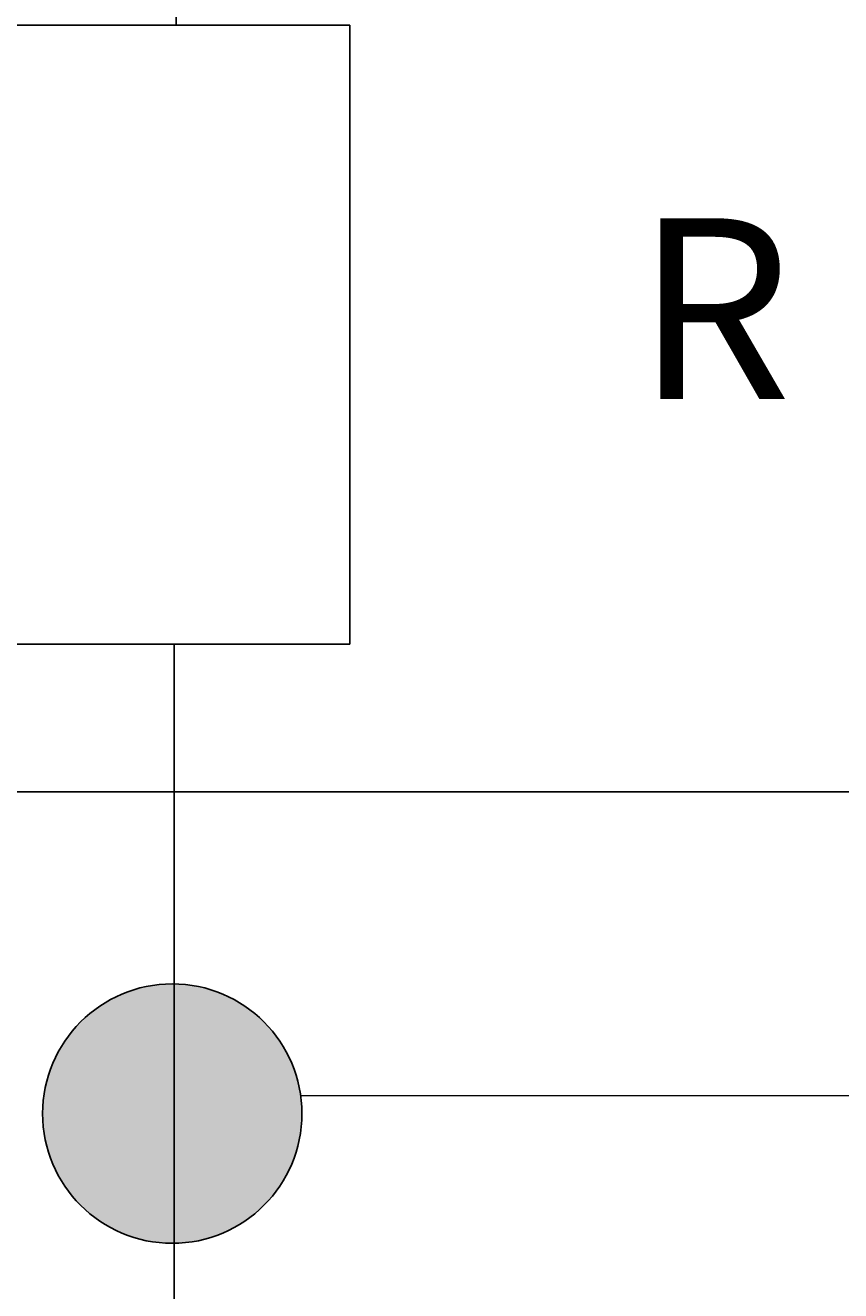
# Model space of a CAD drawing. Units: inches. Extents: x 35362 to 73946, y 43607 to 67532.
# Tile 134 of 134: x 68341 to 69338, y 58575 to 60122. Entities that reach past the tile are written whole.
import ezdxf

# ---------------------------------------------------------------- set-up
doc = ezdxf.new("R2010")
doc.units = ezdxf.units.IN
doc.header["$MEASUREMENT"] = 0
for name, color, linetype, lineweight in [('A-ANNO-DIMS', 2, 'Continuous', 18), ('E-ANNO-TEXT', 5, 'Continuous', 18), ('E-SYMB', 1, 'Continuous', 25), ('E-SYMB-PATT', 1, 'Continuous', 13), ('E-WIRE', 3, 'Continuous', 25)]:
    doc.layers.add(name, color=color, linetype=linetype, lineweight=lineweight)
doc.styles.get("Standard").update_dxf_attribs({"font": 'arial.ttf'})
doc.dimstyles.get("Standard").update_dxf_attribs({"dimtxt": 0.18, "dimasz": 0.18, "dimexe": 0.18, "dimexo": 0.0625, "dimgap": 0.09, "dimtad": 0, "dimtih": 1, "dimtoh": 1, "dimdec": 4, "dimzin": 0, "dimdsep": 46, "dimtxsty": 'Standard', "dimcen": 0.09, "dimadec": 0, "dimazin": 0, "dimtfac": 1, "dimtdec": 4, "dimtofl": 0, "dimtmove": 0, "dimatfit": 3, "dimfxl": 1, "dimtolj": 1, "dimtzin": 0, "dimarcsym": 0})

# ---------------------------------------------------------------- blocks, each defined once
blk = doc.blocks.new('PWR-5V')
for p, q in [((149.83075954589, 1350.920325582869), (-0.0001436721213395, 1075.898385659784)), ((149.83075954589, 833.0941938853575), (149.83075954589, 1350.920325582869)), ((289.9554714129044, 1075.898385659784), (149.83075954589, 1350.920325582869)), ((149.83075954589, 416.3126341884199), (149.83075954589, 833.0941938853575)), ((149.83075954589, 416.3126341884199), (149.83075954589, 0.0003315384019515))]:
    blk.add_line(p, q)
blk = doc.blocks.new('*D8')
at = {"layer": 'A-ANNO-DIMS', "color": 0, "lineweight": -2, "transparency": 16777216}
for p, q in [((66271.28651900003, 65771.51172800003), (73945.82566600003, 65771.51172800003)), ((73945.64566600005, 65771.33172800003), (73945.64566600005, 59737.03093663782)), ((73945.64566600005, 53702.36633900002), (73945.64566600005, 59736.66713036224)), ((72185.70816600003, 53702.18633900003), (73945.82566600003, 53702.18633900003))]:
    blk.add_line(p, q, dxfattribs=at)
at = {"layer": 'A-ANNO-DIMS', "color": 0, "transparency": 16777216}
for points in [[(73945.61566600006, 65771.33172800003), (73945.67566600005, 65771.33172800003), (73945.64566600005, 65771.51172800003)], [(73945.61566600006, 53702.36633900002), (73945.67566600005, 53702.36633900002), (73945.64566600005, 53702.18633900003)]]:
    blk.add_solid(points, dxfattribs=at)
at = {"layer": 'Defpoints', "color": 0, "transparency": 16777216}
for p in [(66271.22401900003, 65771.51172800003), (73945.64566600005, 65771.51172800003), (72185.64566600003, 53702.18633900003)]:
    blk.add_point(p, dxfattribs=at)
at = {"layer": 'A-ANNO-DIMS', "color": 0, "transparency": 16777216, "insert": (73945.64566600005, 59736.84903349999), "char_height": 0.18, "attachment_point": 5}
blk.add_mtext('\\A1;12069', dxfattribs=at)
blk = doc.blocks.new('*D10')
at = {"layer": 'A-ANNO-DIMS', "color": 0, "lineweight": -2, "transparency": 16777216}
for p, q in [((61240.96983600002, 59185.14395700003), (73945.82566600003, 59185.14395700003)), ((73945.64566600005, 59184.96395700003), (73945.64566600005, 56268.51827402935)), ((73945.64566600005, 53351.70866200003), (73945.64566600005, 56268.1543449707)), ((61240.96983600002, 53351.52866200003), (73945.82566600003, 53351.52866200003))]:
    blk.add_line(p, q, dxfattribs=at)
at = {"layer": 'A-ANNO-DIMS', "color": 0, "transparency": 16777216}
for points in [[(73945.61566600006, 59184.96395700003), (73945.67566600005, 59184.96395700003), (73945.64566600005, 59185.14395700003)], [(73945.61566600006, 53351.70866200003), (73945.67566600005, 53351.70866200003), (73945.64566600005, 53351.52866200003)]]:
    blk.add_solid(points, dxfattribs=at)
at = {"layer": 'Defpoints', "color": 0, "transparency": 16777216}
for p in [(61240.90733600002, 59185.14395700003), (61240.90733600002, 53351.52866200003), (73945.64566600005, 53351.52866200003)]:
    blk.add_point(p, dxfattribs=at)
at = {"layer": 'A-ANNO-DIMS', "color": 0, "transparency": 16777216, "insert": (73945.64566600005, 56268.33630949999), "char_height": 0.18, "attachment_point": 5}
blk.add_mtext('\\A1;5834', dxfattribs=at)
blk = doc.blocks.new('*D69')
at = {"layer": 'A-ANNO-DIMS', "color": 0, "lineweight": -2, "transparency": 16777216}
for p, q in [((68320.870762, 60122.408832), (68320.870762, 67531.691728)), ((68321.050762, 67531.51172799998), (69913.30289879469, 67531.51172799998)), ((71506.482539, 67531.51172799998), (69914.23040220531, 67531.51172799998)), ((71506.662539, 59451.647447), (71506.662539, 67531.691728))]:
    blk.add_line(p, q, dxfattribs=at)
at = {"layer": 'A-ANNO-DIMS', "color": 0, "transparency": 16777216}
for points in [[(68321.050762, 67531.541728), (68321.050762, 67531.481728), (68320.870762, 67531.51172799998)], [(71506.482539, 67531.541728), (71506.482539, 67531.481728), (71506.662539, 67531.51172799998)]]:
    blk.add_solid(points, dxfattribs=at)
at = {"layer": 'Defpoints', "color": 0, "transparency": 16777216}
for p in [(71506.662539, 67531.51172799998), (68320.870762, 60122.346332), (71506.662539, 59451.584947)]:
    blk.add_point(p, dxfattribs=at)
at = {"layer": 'A-ANNO-DIMS', "color": 0, "transparency": 16777216, "insert": (69913.76665050001, 67531.51172799998), "char_height": 0.18, "attachment_point": 5}
blk.add_mtext('\\A1;3185.8', dxfattribs=at)
blk = doc.blocks.new('*D70')
at = {"layer": 'A-ANNO-DIMS', "color": 0, "lineweight": -2, "transparency": 16777216}
for p, q in [((60785.27513900002, 64923.75242000003), (73945.82566600003, 64923.75242000003)), ((73945.64566600005, 64923.57242000003), (73945.64566600005, 62054.63015302935)), ((73945.64566600005, 59185.32395700003), (73945.64566600005, 62054.26622397069)), ((61240.96983600002, 59185.14395700003), (73945.82566600003, 59185.14395700003))]:
    blk.add_line(p, q, dxfattribs=at)
at = {"layer": 'A-ANNO-DIMS', "color": 0, "transparency": 16777216}
for points in [[(73945.61566600006, 64923.57242000003), (73945.67566600005, 64923.57242000003), (73945.64566600005, 64923.75242000003)], [(73945.61566600006, 59185.32395700003), (73945.67566600005, 59185.32395700003), (73945.64566600005, 59185.14395700003)]]:
    blk.add_solid(points, dxfattribs=at)
at = {"layer": 'Defpoints', "color": 0, "transparency": 16777216}
for p in [(60785.21263900002, 64923.75242000003), (73945.64566600005, 64923.75242000003), (61240.90733600002, 59185.14395700003)]:
    blk.add_point(p, dxfattribs=at)
at = {"layer": 'A-ANNO-DIMS', "color": 0, "transparency": 16777216, "insert": (73945.64566600005, 62054.44818849999), "char_height": 0.18, "attachment_point": 5}
blk.add_mtext('\\A1;5738.6', dxfattribs=at)
blk = doc.blocks.new('*D71')
at = {"layer": 'A-ANNO-DIMS', "color": 0, "lineweight": -2, "transparency": 16777216}
for p, q in [((63159.24181700003, 64828.55626700002), (73945.82566600003, 64828.55626700002)), ((73945.64566600005, 64828.37626700002), (73945.64566600005, 62007.03207652936)), ((73945.64566600005, 59185.32395700003), (73945.64566600005, 62006.6681474707)), ((61240.96983600002, 59185.14395700003), (73945.82566600003, 59185.14395700003))]:
    blk.add_line(p, q, dxfattribs=at)
at = {"layer": 'A-ANNO-DIMS', "color": 0, "transparency": 16777216}
for points in [[(73945.61566600006, 64828.37626700002), (73945.67566600005, 64828.37626700002), (73945.64566600005, 64828.55626700002)], [(73945.61566600006, 59185.32395700003), (73945.67566600005, 59185.32395700003), (73945.64566600005, 59185.14395700003)]]:
    blk.add_solid(points, dxfattribs=at)
at = {"layer": 'Defpoints', "color": 0, "transparency": 16777216}
for p in [(63159.17931700003, 64828.55626700002), (73945.64566600005, 64828.55626700002), (61240.90733600002, 59185.14395700003)]:
    blk.add_point(p, dxfattribs=at)
at = {"layer": 'A-ANNO-DIMS', "color": 0, "transparency": 16777216, "insert": (73945.64566600005, 62006.85011199999), "char_height": 0.18, "attachment_point": 5}
blk.add_mtext('\\A1;5643.4', dxfattribs=at)

msp = doc.modelspace()

# ---------------------------------------------------------------- hatches: boundary and pattern name
at = {"layer": 'E-SYMB-PATT'}
h = msp.add_hatch(color=256, dxfattribs=at)
h.dxf.hatch_style = 1
h.paths.add_polyline_path([(68522.99328781641, 58950.10275888999, 0.4183931940818975), (68362.12749647925, 58791.51297351146, 0.4183931940818975), (68522.99328781641, 58632.92318813292)])
h.paths.add_polyline_path([(68522.99328781641, 58950.10275888999), (68522.99328781641, 58632.92318813292, 0.4100462469397049), (68679.33926925441, 58791.51297351146, 0.4100462469397049)])

# ---------------------------------------------------------------- linework, layer by layer
at = {"layer": 'E-SYMB'}
for p, q in [((68522.99328781641, 59095.61234402943), (68522.99328781641, 59365.72803786365)), ((68518.41798978415, 58950.10195847468), (68518.41798978415, 58949.41573521363)), ((68522.99328781641, 58637.39433361782), (68522.99328781641, 58632.92318813292))]:
    msp.add_line(p, q, dxfattribs=at)
msp.add_lwpolyline([(68320.87076221016, 60122.34633153839), (68737.80188109005, 60122.34633153839), (68737.80188109005, 59365.72803786365), (68320.87076221016, 59365.72803786365)], close=True, dxfattribs=at)
msp.add_circle((68520.73338286683, 58791.51297351146), 158.6058863875805, dxfattribs=at)
at = {"layer": 'E-WIRE'}
for p, q in [((68522.99328781641, 58468.38124608586), (68522.99328781641, 59095.61234402943)), ((70135.80528894292, 58812.79476317562), (68677.76702326702, 58813.78993424351))]:
    msp.add_line(p, q, dxfattribs=at)

# ---------------------------------------------------------------- block references
at = {"layer": 'E-SYMB'}
msp.add_blockref('PWR-5V', (68375.605, 60122.346), dxfattribs=at)

# ---------------------------------------------------------------- texts
at = {"layer": 'E-ANNO-TEXT'}
msp.add_text('R', height=220.8659825270206, dxfattribs=at).set_placement((69087.11378477843, 59665.4646863401))

# ---------------------------------------------------------------- dimensions: what is measured, and where the dimension line sits
at = {"layer": 'A-ANNO-DIMS'}
dim = msp.add_linear_dim(base=(71506.662539, 67531.51172799998), p1=(68320.870762, 60122.346332), p2=(71506.662539, 59451.584947), dimstyle='Standard', override={"dimdec": 1, "dimlfac": 1, "dimrnd": 0, "dimzin": 0, "dimdsep": 46, "dimlunit": 2}, dxfattribs=at)
dim.commit()
dim.dimension.update_dxf_attribs({"geometry": '*D69', "text_midpoint": (69913.76665050001, 67531.51172799998)})
for base, p1, p2, override, picture, middle in [((73945.64566600005, 65771.51172800003), (72185.645666, 53702.186339), (66271.224019, 65771.51172799998), {"dimdec": 0, "dimlfac": 1, "dimrnd": 0, "dimzin": 0, "dimdsep": 46, "dimlunit": 2}, '*D8', (73945.64566600005, 59736.84903349999)), ((73945.64566600005, 64923.75242000003), (61240.907336, 59185.14395699999), (60785.21263899999, 64923.75241999999), {"dimdec": 1, "dimlfac": 1, "dimrnd": 0, "dimzin": 0, "dimdsep": 46, "dimlunit": 2}, '*D70', (73945.64566600005, 62054.44818849999)), ((73945.64566600005, 64828.55626700002), (61240.907336, 59185.14395699999), (63159.179317, 64828.556267), {"dimdec": 1, "dimlfac": 1, "dimrnd": 0, "dimzin": 0, "dimdsep": 46, "dimlunit": 2}, '*D71', (73945.64566600005, 62006.85011199999)), ((73945.64566600005, 53351.52866200003), (61240.907336, 59185.14395699999), (61240.907336, 53351.52866199999), {"dimdec": 0, "dimlfac": 1, "dimrnd": 0, "dimzin": 0, "dimdsep": 46, "dimlunit": 2}, '*D10', (73945.64566600005, 56268.33630949999))]:
    dim = msp.add_linear_dim(base=base, p1=p1, p2=p2, angle=90, dimstyle='Standard', override=override, dxfattribs=at)
    dim.commit()
    dim.dimension.update_dxf_attribs({"geometry": picture, "text_midpoint": middle})

doc.saveas('drawing.dxf')
